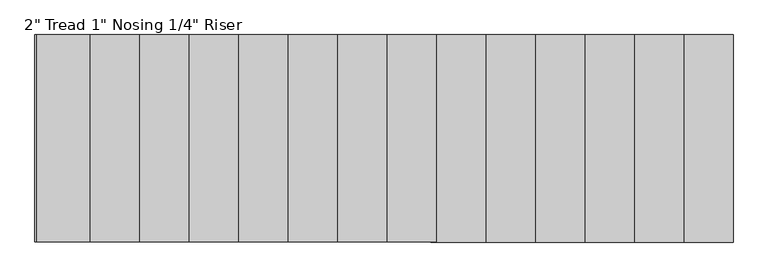
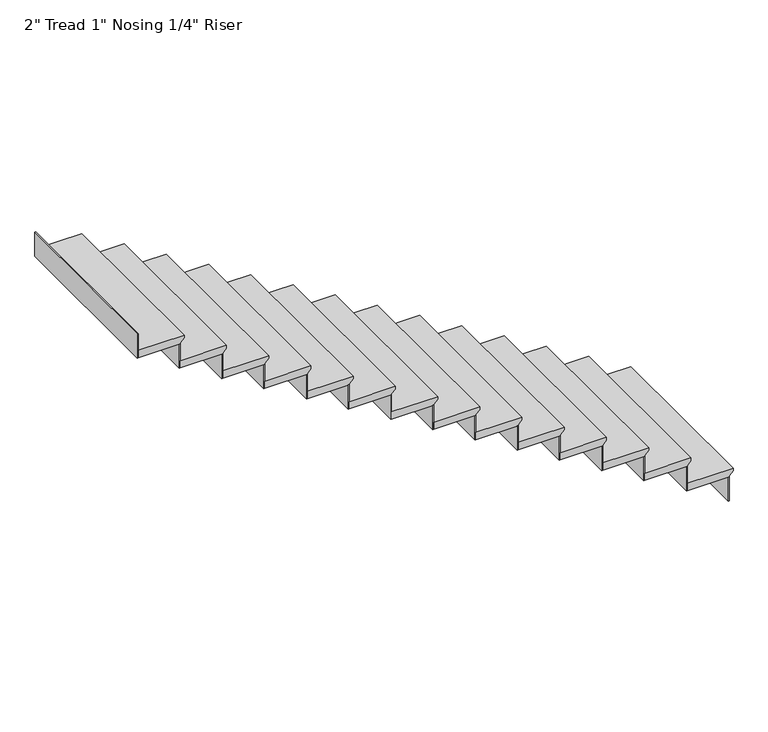
"""IFC4 building model written with IfcOpenShell, lengths in millimetres: stair flight geometry."""

from ifc_helpers import new_model, si_unit, frame, origin, place, context, project, spatial, polyline, outline, extrude, source, transform, mapped, element, save


def stair_flight_7a186021(model_context):
    return source(origin(), model_context, "Body", "SweptSolid", [
        extrude(outline(polyline([(1185.3333333, -1706.7886283), (1185.3333333, -2011.5886283), (1134.5333333, -2011.5886283), (1134.5333333, -1732.1886283), (1140.8833333, -1732.1886283), (1166.2833333, -1706.7886283), (1185.3333333, -1706.7886283)])), frame((0.0, 4034.5574946, 0.0), z_axis=(0.0, 1.0, 0.0), x_axis=(0.0, 0.0, 1.0)), (0.0, 0.0, 1.0), 1172.2503627),
        extrude(outline(polyline([(-1738.5386283, 5206.8078573), (-1732.1886283, 5206.8078573), (-1732.1886283, 4034.5574946), (-1738.5386283, 4034.5574946), (-1738.5386283, 5206.8078573)])), frame((0.0, 0.0, 965.2), z_axis=(0.0, 0.0, 1.0), x_axis=(1.0, 0.0, 0.0)), (0.0, 0.0, 1.0), 169.3333333),
        extrude(outline(polyline([(-2017.9386283, 5206.8078573), (-2011.5886283, 5206.8078573), (-2011.5886283, 4034.5574946), (-2017.9386283, 4034.5574946), (-2017.9386283, 5206.8078573)])), frame((0.0, 0.0, 1134.5333333), z_axis=(0.0, 0.0, 1.0), x_axis=(1.0, 0.0, 0.0)), (0.0, 0.0, 1.0), 169.3333333),
        extrude(outline(polyline([(1354.6666667, -1986.1886283), (1354.6666667, -2290.9886283), (1303.8666667, -2290.9886283), (1303.8666667, -2011.5886283), (1310.2166667, -2011.5886283), (1335.6166667, -1986.1886283), (1354.6666667, -1986.1886283)])), frame((0.0, 4034.5574946, 0.0), z_axis=(0.0, 1.0, 0.0), x_axis=(0.0, 0.0, 1.0)), (0.0, 0.0, 1.0), 1172.2503627),
        extrude(outline(polyline([(-2297.3386283, 5206.8078573), (-2290.9886283, 5206.8078573), (-2290.9886283, 4034.5574946), (-2297.3386283, 4034.5574946), (-2297.3386283, 5206.8078573)])), frame((0.0, 0.0, 1303.8666667), z_axis=(0.0, 0.0, 1.0), x_axis=(1.0, 0.0, 0.0)), (0.0, 0.0, 1.0), 169.3333333),
        extrude(outline(polyline([(1524.0, -2265.5886283), (1524.0, -2570.3886283), (1473.2, -2570.3886283), (1473.2, -2290.9886283), (1479.55, -2290.9886283), (1504.95, -2265.5886283), (1524.0, -2265.5886283)])), frame((0.0, 4034.5574946, 0.0), z_axis=(0.0, 1.0, 0.0), x_axis=(0.0, 0.0, 1.0)), (0.0, 0.0, 1.0), 1172.2503627),
        extrude(outline(polyline([(-2576.7386283, 5206.8078573), (-2570.3886283, 5206.8078573), (-2570.3886283, 4034.5574946), (-2576.7386283, 4034.5574946), (-2576.7386283, 5206.8078573)])), frame((0.0, 0.0, 1473.2), z_axis=(0.0, 0.0, 1.0), x_axis=(1.0, 0.0, 0.0)), (0.0, 0.0, 1.0), 169.3333333),
        extrude(outline(polyline([(1693.3333333, -2544.9886283), (1693.3333333, -2849.7886283), (1642.5333333, -2849.7886283), (1642.5333333, -2570.3886283), (1648.8833333, -2570.3886283), (1674.2833333, -2544.9886283), (1693.3333333, -2544.9886283)])), frame((0.0, 4034.5574946, 0.0), z_axis=(0.0, 1.0, 0.0), x_axis=(0.0, 0.0, 1.0)), (0.0, 0.0, 1.0), 1172.2503627),
        extrude(outline(polyline([(-2856.1386283, 5206.8078573), (-2849.7886283, 5206.8078573), (-2849.7886283, 4034.5574946), (-2856.1386283, 4034.5574946), (-2856.1386283, 5206.8078573)])), frame((0.0, 0.0, 1642.5333333), z_axis=(0.0, 0.0, 1.0), x_axis=(1.0, 0.0, 0.0)), (0.0, 0.0, 1.0), 169.3333333),
        extrude(outline(polyline([(1862.6666667, -2824.3886283), (1862.6666667, -3129.1886283), (1811.8666667, -3129.1886283), (1811.8666667, -2849.7886283), (1818.2166667, -2849.7886283), (1843.6166667, -2824.3886283), (1862.6666667, -2824.3886283)])), frame((0.0, 4034.5574946, 0.0), z_axis=(0.0, 1.0, 0.0), x_axis=(0.0, 0.0, 1.0)), (0.0, 0.0, 1.0), 1172.2503627),
        extrude(outline(polyline([(-3135.5386283, 5206.8078573), (-3129.1886283, 5206.8078573), (-3129.1886283, 4034.5574946), (-3135.5386283, 4034.5574946), (-3135.5386283, 5206.8078573)])), frame((0.0, 0.0, 1811.8666667), z_axis=(0.0, 0.0, 1.0), x_axis=(1.0, 0.0, 0.0)), (0.0, 0.0, 1.0), 169.3333333),
        extrude(outline(polyline([(2032.0, -3103.7886283), (2032.0, -3408.5886283), (1981.2, -3408.5886283), (1981.2, -3129.1886283), (1987.55, -3129.1886283), (2012.95, -3103.7886283), (2032.0, -3103.7886283)])), frame((0.0, 4034.5574946, 0.0), z_axis=(0.0, 1.0, 0.0), x_axis=(0.0, 0.0, 1.0)), (0.0, 0.0, 1.0), 1172.2503627),
        extrude(outline(polyline([(-3414.9386283, 5206.8078573), (-3408.5886283, 5206.8078573), (-3408.5886283, 4034.5574946), (-3414.9386283, 4034.5574946), (-3414.9386283, 5206.8078573)])), frame((0.0, 0.0, 1981.2), z_axis=(0.0, 0.0, 1.0), x_axis=(1.0, 0.0, 0.0)), (0.0, 0.0, 1.0), 169.3333333),
        extrude(outline(polyline([(2201.3333333, -3383.1886283), (2201.3333333, -3687.9886283), (2150.5333333, -3687.9886283), (2150.5333333, -3408.5886283), (2156.8833333, -3408.5886283), (2182.2833333, -3383.1886283), (2201.3333333, -3383.1886283)])), frame((0.0, 4034.5574946, 0.0), z_axis=(0.0, 1.0, 0.0), x_axis=(0.0, 0.0, 1.0)), (0.0, 0.0, 1.0), 1172.2503627),
        extrude(outline(polyline([(-3694.3386283, 5206.8078573), (-3687.9886283, 5206.8078573), (-3687.9886283, 4034.5574946), (-3694.3386283, 4034.5574946), (-3694.3386283, 5206.8078573)])), frame((0.0, 0.0, 2150.5333333), z_axis=(0.0, 0.0, 1.0), x_axis=(1.0, 0.0, 0.0)), (0.0, 0.0, 1.0), 169.3333333),
        extrude(outline(polyline([(2370.6666667, -3662.5886283), (2370.6666667, -3967.3886283), (2319.8666667, -3967.3886283), (2319.8666667, -3687.9886283), (2326.2166667, -3687.9886283), (2351.6166667, -3662.5886283), (2370.6666667, -3662.5886283)])), frame((0.0, 4034.5574946, 0.0), z_axis=(0.0, 1.0, 0.0), x_axis=(0.0, 0.0, 1.0)), (0.0, 0.0, 1.0), 1172.2503627),
        extrude(outline(polyline([(-3973.7386283, 5206.8078573), (-3967.3886283, 5206.8078573), (-3967.3886283, 4034.5574946), (-3973.7386283, 4034.5574946), (-3973.7386283, 5206.8078573)])), frame((0.0, 0.0, 2319.8666667), z_axis=(0.0, 0.0, 1.0), x_axis=(1.0, 0.0, 0.0)), (0.0, 0.0, 1.0), 169.3333333),
        extrude(outline(polyline([(2540.0, -3941.9886283), (2540.0, -4246.7886283), (2489.2, -4246.7886283), (2489.2, -3967.3886283), (2495.55, -3967.3886283), (2520.95, -3941.9886283), (2540.0, -3941.9886283)])), frame((0.0, 4034.5574946, 0.0), z_axis=(0.0, 1.0, 0.0), x_axis=(0.0, 0.0, 1.0)), (0.0, 0.0, 1.0), 1172.2503627),
        extrude(outline(polyline([(-4253.1386283, 5206.8078573), (-4246.7886283, 5206.8078573), (-4246.7886283, 4034.5574946), (-4253.1386283, 4034.5574946), (-4253.1386283, 5206.8078573)])), frame((0.0, 0.0, 2489.2), z_axis=(0.0, 0.0, 1.0), x_axis=(1.0, 0.0, 0.0)), (0.0, 0.0, 1.0), 169.3333333),
        extrude(outline(polyline([(2709.3333333, -4221.3886283), (2709.3333333, -4526.1886283), (2658.5333333, -4526.1886283), (2658.5333333, -4246.7886283), (2664.8833333, -4246.7886283), (2690.2833333, -4221.3886283), (2709.3333333, -4221.3886283)])), frame((0.0, 4034.5574946, 0.0), z_axis=(0.0, 1.0, 0.0), x_axis=(0.0, 0.0, 1.0)), (0.0, 0.0, 1.0), 1172.2503627),
        extrude(outline(polyline([(-4532.5386283, 5206.8078573), (-4526.1886283, 5206.8078573), (-4526.1886283, 4034.5574946), (-4532.5386283, 4034.5574946), (-4532.5386283, 5206.8078573)])), frame((0.0, 0.0, 2658.5333333), z_axis=(0.0, 0.0, 1.0), x_axis=(1.0, 0.0, 0.0)), (0.0, 0.0, 1.0), 169.3333333),
        extrude(outline(polyline([(2878.6666667, -4500.7886283), (2878.6666667, -4805.5886283), (2827.8666667, -4805.5886283), (2827.8666667, -4526.1886283), (2834.2166667, -4526.1886283), (2859.6166667, -4500.7886283), (2878.6666667, -4500.7886283)])), frame((0.0, 4034.5574946, 0.0), z_axis=(0.0, 1.0, 0.0), x_axis=(0.0, 0.0, 1.0)), (0.0, 0.0, 1.0), 1172.2503627),
        extrude(outline(polyline([(-4811.9386283, 5206.8078573), (-4805.5886283, 5206.8078573), (-4805.5886283, 4034.5574946), (-4811.9386283, 4034.5574946), (-4811.9386283, 5206.8078573)])), frame((0.0, 0.0, 2827.8666667), z_axis=(0.0, 0.0, 1.0), x_axis=(1.0, 0.0, 0.0)), (0.0, 0.0, 1.0), 169.3333333),
        extrude(outline(polyline([(3048.0, -4780.1886283), (3048.0, -5084.9886283), (2997.2, -5084.9886283), (2997.2, -4805.5886283), (3003.55, -4805.5886283), (3028.95, -4780.1886283), (3048.0, -4780.1886283)])), frame((0.0, 4034.5574946, 0.0), z_axis=(0.0, 1.0, 0.0), x_axis=(0.0, 0.0, 1.0)), (0.0, 0.0, 1.0), 1172.2503627),
        extrude(outline(polyline([(-5091.3386283, 5206.8078573), (-5084.9886283, 5206.8078573), (-5084.9886283, 4034.5574946), (-5091.3386283, 4034.5574946), (-5091.3386283, 5206.8078573)])), frame((0.0, 0.0, 2997.2), z_axis=(0.0, 0.0, 1.0), x_axis=(1.0, 0.0, 0.0)), (0.0, 0.0, 1.0), 169.3333333),
        extrude(outline(polyline([(3217.3333333, -5059.5886283), (3217.3333333, -5364.3886283), (3166.5333333, -5364.3886283), (3166.5333333, -5084.9886283), (3172.8833333, -5084.9886283), (3198.2833333, -5059.5886283), (3217.3333333, -5059.5886283)])), frame((0.0, 4034.5574946, 0.0), z_axis=(0.0, 1.0, 0.0), x_axis=(0.0, 0.0, 1.0)), (0.0, 0.0, 1.0), 1172.2503627),
        extrude(outline(polyline([(-5370.7386283, 5206.8078573), (-5364.3886283, 5206.8078573), (-5364.3886283, 4034.5574946), (-5370.7386283, 4034.5574946), (-5370.7386283, 5206.8078573)])), frame((0.0, 0.0, 3166.5333333), z_axis=(0.0, 0.0, 1.0), x_axis=(1.0, 0.0, 0.0)), (0.0, 0.0, 1.0), 169.3333333),
        extrude(outline(polyline([(-5650.1386283, 5206.8078573), (-5643.7886283, 5206.8078573), (-5643.7886283, 4034.5574946), (-5650.1386283, 4034.5574946), (-5650.1386283, 5206.8078573)])), frame((0.0, 0.0, 3335.8666667), z_axis=(0.0, 0.0, 1.0), x_axis=(1.0, 0.0, 0.0)), (0.0, 0.0, 1.0), 169.3333333),
        extrude(outline(polyline([(3386.6666667, -5338.9886283), (3386.6666667, -5643.7886283), (3335.8666667, -5643.7886283), (3335.8666667, -5364.3886283), (3342.2166667, -5364.3886283), (3367.6166667, -5338.9886283), (3386.6666667, -5338.9886283)])), frame((0.0, 4034.5574946, 0.0), z_axis=(0.0, 1.0, 0.0), x_axis=(0.0, 0.0, 1.0)), (0.0, 0.0, 1.0), 1172.2503627),
    ])


if __name__ == "__main__":
    model = new_model("IFC4")
    model_context = context("Model", 3, world=origin())
    ifc_project = project(units=[si_unit("LENGTHUNIT", "METRE", prefix="MILLI")], contexts=[model_context])
    site = spatial("IfcSite", under=ifc_project)
    building = spatial("IfcBuilding", under=site)
    placement = place(None, origin())
    stair_flight_shape = stair_flight_7a186021(model_context)
    element("IfcStairFlight", 1, ObjectType="2\" Tread 1\" Nosing 1/4\" Riser", at=placement, inside=building, context=model_context, shape_type="MappedRepresentation", body=[
        mapped(stair_flight_shape, transform((0.0, 0.0, 0.0), x_axis=(1.0, 0.0, 0.0), y_axis=(0.0, 1.0, 0.0), z_axis=(0.0, 0.0, 1.0))),
    ])
    save(model, "model.ifc")
